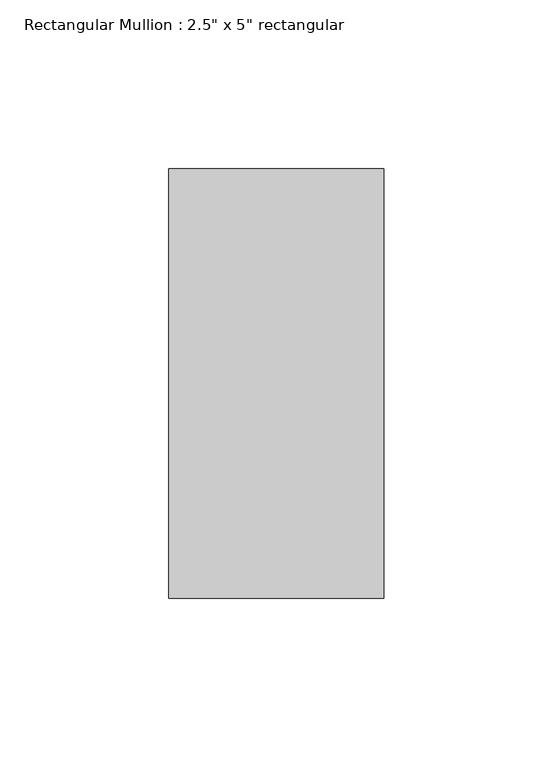
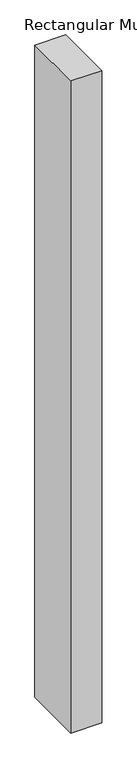
"""IFC4 building model written with IfcOpenShell, lengths in millimetres: member geometry."""

from ifc_helpers import new_model, si_unit, frame, origin, place, context, project, spatial, polyline, outline, extrude, source, transform, mapped, element, save


def member_66888762(model_context):
    return source(origin(), model_context, "Body", "SweptSolid", [
        extrude(outline(polyline([(0.0, 63.5), (0.0, -63.5), (-63.5, -63.5), (-63.5, 63.5), (0.0, 63.5)])), frame((0.0, 0.0, -1408.8373989), z_axis=(0.0, 0.0, 1.0), x_axis=(1.0, 0.0, 0.0)), (0.0, 0.0, 1.0), 1408.8373989),
    ])


if __name__ == "__main__":
    model = new_model("IFC4")
    model_context = context("Model", 3, world=origin())
    ifc_project = project(units=[si_unit("LENGTHUNIT", "METRE", prefix="MILLI")], contexts=[model_context])
    site = spatial("IfcSite", under=ifc_project)
    building = spatial("IfcBuilding", under=site)
    placement = place(None, origin())
    member_shape = member_66888762(model_context)
    element("IfcMember", 1, ObjectType="Rectangular Mullion : 2.5\" x 5\" rectangular", at=placement, inside=building, context=model_context, shape_type="MappedRepresentation", body=[
        mapped(member_shape, transform((0.0, 0.0, 0.0), x_axis=(1.0, 0.0, 0.0), y_axis=(0.0, 1.0, 0.0), z_axis=(0.0, 0.0, 1.0))),
    ])
    save(model, "model.ifc")

# Revit data of these elements
# Type "Rectangular Mullion : 2.5\" x 5\" rectangular"
#   built-in parameter 1007304 = 0.416667 (stored number, unit not read)
#   built-in parameter 1007301 = 0.104167 (stored number, unit not read)
#   built-in parameter 1007300 = 0.104167 (stored number, unit not read)
# Element 1 (IfcMember, "Rectangular Mullion : 2.5\" x 5\" rectangular")
#   Materials on its faces: "Aluminum"
# Materials
#   "Aluminum": class "Metal", colour RGB 247 247 247, transparency 0, Description = "Aluminum 6061", Cost = 0
